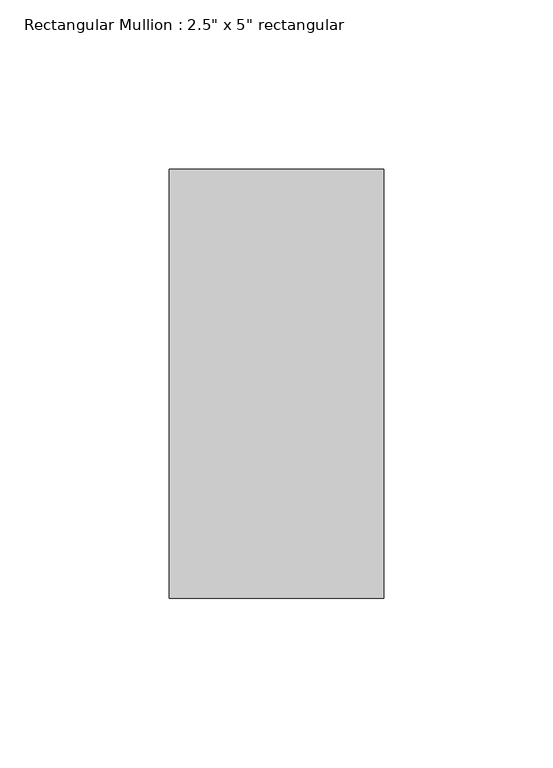
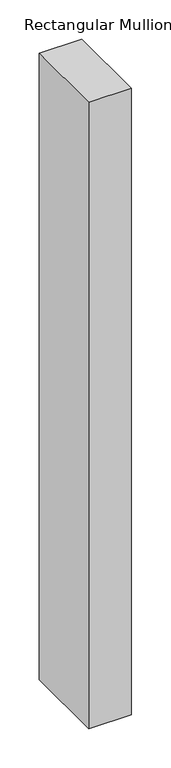
"""IFC4 building model written with IfcOpenShell, lengths in millimetres: member geometry."""

from ifc_helpers import new_model, si_unit, frame, origin, place, context, project, spatial, polyline, outline, extrude, source, transform, mapped, element, save


def member_a80f276a(model_context):
    return source(origin(), model_context, "Body", "SweptSolid", [
        extrude(outline(polyline([(0.0, 63.5), (0.0, -63.5), (-63.5, -63.5), (-63.5, 63.5), (0.0, 63.5)])), frame((0.0, 0.0, -980.0145651), z_axis=(0.0, 0.0, 1.0), x_axis=(1.0, 0.0, 0.0)), (0.0, 0.0, 1.0), 980.0145651),
    ])


if __name__ == "__main__":
    model = new_model("IFC4")
    model_context = context("Model", 3, world=origin())
    ifc_project = project(units=[si_unit("LENGTHUNIT", "METRE", prefix="MILLI")], contexts=[model_context])
    site = spatial("IfcSite", under=ifc_project)
    building = spatial("IfcBuilding", under=site)
    placement = place(None, origin())
    member_shape = member_a80f276a(model_context)
    element("IfcMember", 1, ObjectType="Rectangular Mullion : 2.5\" x 5\" rectangular", at=placement, inside=building, context=model_context, shape_type="MappedRepresentation", body=[
        mapped(member_shape, transform((0.0, 0.0, 0.0), x_axis=(1.0, 0.0, 0.0), y_axis=(0.0, 1.0, 0.0), z_axis=(0.0, 0.0, 1.0))),
    ])
    save(model, "model.ifc")

# Revit data of these elements
# Type "Rectangular Mullion : 2.5\" x 5\" rectangular"
#   built-in parameter 1007304 = 0.416667 (stored number, unit not read)
#   built-in parameter 1007301 = 0.104167 (stored number, unit not read)
#   built-in parameter 1007300 = 0.104167 (stored number, unit not read)
# Element 1 (IfcMember, "Rectangular Mullion : 2.5\" x 5\" rectangular")
#   Materials on its faces: "Aluminum"
# Materials
#   "Aluminum": class "Metal", colour RGB 247 247 247, transparency 0, Description = "Aluminum 6061", Cost = 0
